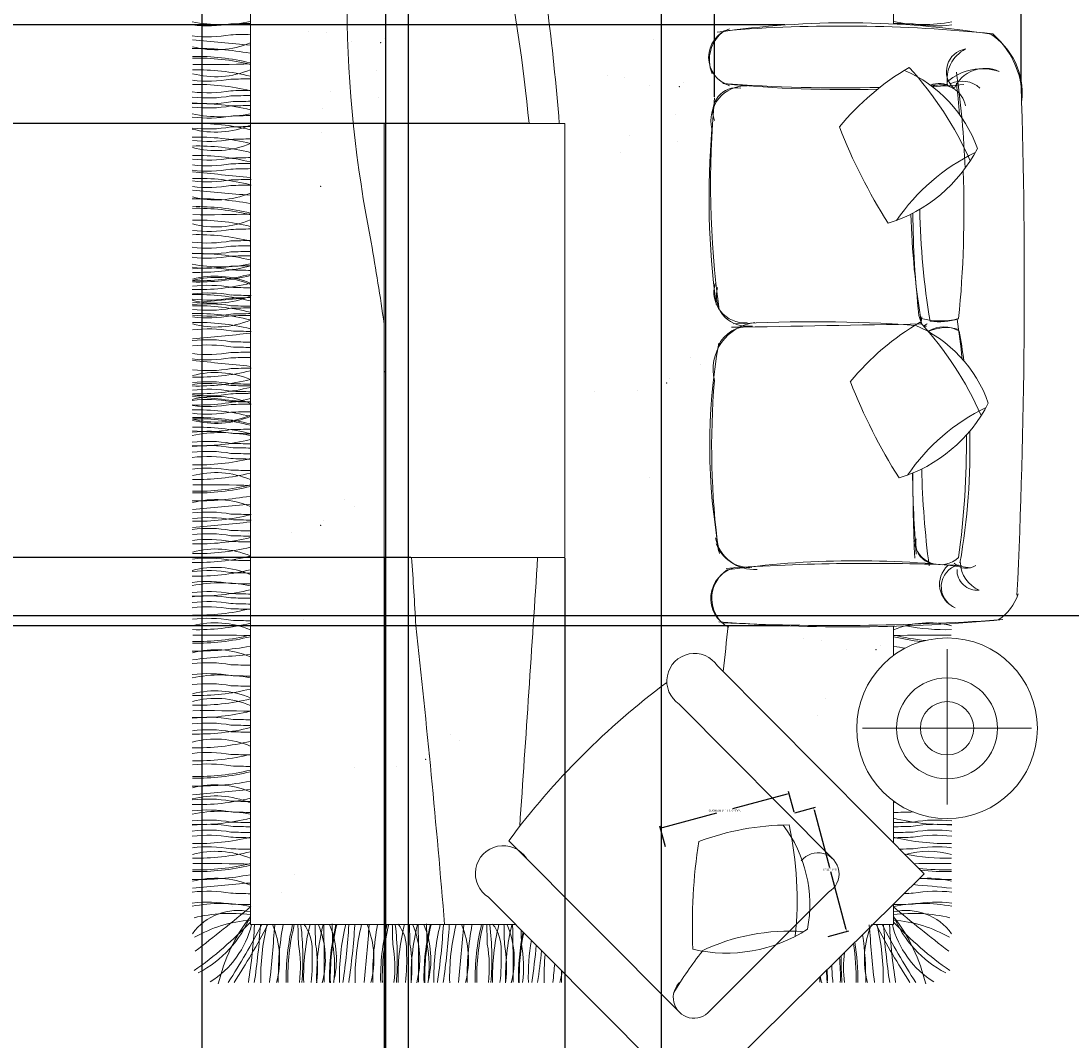
# Model space of a CAD drawing. Units: inches. Extents: x 503 to 1084, y -605 to 132.
# Tile 9 of 14: x 882 to 974, y -318 to -230. Entities that reach past the tile are written whole.
import ezdxf

# ---------------------------------------------------------------- set-up
doc = ezdxf.new("R2010")
doc.units = ezdxf.units.IN
doc.header["$MEASUREMENT"] = 0
doc.layers.add('A-ANNO-DIMS', color=7, linetype='Continuous', lineweight=18)
doc.layers.add('furniture', color=50, linetype='Continuous', lineweight=13, transparency=0.8)
doc.styles.get("Standard").update_dxf_attribs({"font": 'arial.ttf'})
doc.dimstyles.get("Standard").update_dxf_attribs({"dimtxt": 0.18, "dimasz": 0.18, "dimexe": 0.18, "dimexo": 0.0625, "dimgap": 0.09, "dimtad": 0, "dimtih": 1, "dimtoh": 1, "dimdec": 1, "dimzin": 0, "dimdsep": 46, "dimlunit": 4, "dimtxsty": 'Standard', "dimcen": 0.09, "dimadec": 0, "dimazin": 0, "dimtfac": 1, "dimtdec": 1, "dimtofl": 0, "dimtmove": 0, "dimatfit": 3, "dimfxl": 1, "dimtolj": 1, "dimtzin": 0, "dimarcsym": 0})

# ---------------------------------------------------------------- blocks, each defined once
blk = doc.blocks.new('CUSHION-SCATTER')
for centre, radius, start, end in [((-0.355, -5.979), 11.599, 64.45006, 111.76991), ((17.467, -0.489), 22.747, 165.30685, 185.5663), ((-5.995, -25.402), 30.717, 69.08153, 87.27682), ((-7.72, 0.481), 12.999, 332.0126, 17.9429), ((21.395, -1.669), 17.594, 160.90051, 190.65125), ((14.361, 41.881), 48.668, 246.33709, 257.41765)]:
    blk.add_arc(centre, radius, start, end)
blk = doc.blocks.new('*D30')
at = {"layer": 'A-ANNO-DIMS', "color": 0, "lineweight": -2, "transparency": 16777216}
for p, q in [((949.077, -296.859), (944.325, -298.132)), ((949.685, -298.435), (949.204, -296.639)), ((938.207, -299.772), (942.958, -298.499)), ((938.468, -301.441), (937.986, -299.645))]:
    blk.add_line(p, q, dxfattribs=at)
at = {"layer": 'A-ANNO-DIMS', "color": 0, "transparency": 16777216}
for points in [[(949.069, -296.83), (949.084, -296.888), (949.251, -296.813)], [(938.199, -299.743), (938.214, -299.801), (938.033, -299.818)]]:
    blk.add_solid(points, dxfattribs=at)
at = {"layer": 'Defpoints', "color": 0, "transparency": 16777216}
for p in [(949.251, -296.813), (949.701, -298.495), (938.484, -301.501)]:
    blk.add_point(p, dxfattribs=at)
at = {"layer": 'A-ANNO-DIMS', "color": 0, "transparency": 16777216, "insert": (943.642, -298.315), "char_height": 0.18, "attachment_point": 5}
blk.add_mtext('\\A1;CUSHION 0\'-11 1/2" TYP.', dxfattribs=at)
blk = doc.blocks.new('*D31')
at = {"layer": 'A-ANNO-DIMS', "color": 0, "lineweight": -2, "transparency": 16777216}
for p, q in [((949.762, -298.479), (951.558, -297.998)), ((951.431, -298.218), (952.78, -303.255)), ((954.227, -308.655), (952.878, -303.618)), ((952.651, -309.263), (954.448, -308.782))]:
    blk.add_line(p, q, dxfattribs=at)
at = {"layer": 'A-ANNO-DIMS', "color": 0, "transparency": 16777216}
for points in [[(951.46, -298.211), (951.402, -298.226), (951.384, -298.044)], [(954.256, -308.647), (954.198, -308.663), (954.274, -308.829)]]:
    blk.add_solid(points, dxfattribs=at)
at = {"layer": 'Defpoints', "color": 0, "transparency": 16777216}
for p in [(949.701, -298.495), (954.274, -308.829), (952.591, -309.279)]:
    blk.add_point(p, dxfattribs=at)
at = {"layer": 'A-ANNO-DIMS', "color": 0, "transparency": 16777216, "insert": (952.829, -303.437), "char_height": 0.18, "attachment_point": 5}
blk.add_mtext('\\A1;0\'-11" TYP.', dxfattribs=at)
blk = doc.blocks.new('*D45')
at = {"layer": 'A-ANNO-DIMS', "color": 0, "lineweight": -2, "transparency": 16777216}
for p, q in [((844.089, -354.753), (844.089, 43.514)), ((844.269, 43.334), (879.759, 43.334)), ((915.909, 43.334), (880.418, 43.334)), ((916.089, -354.753), (916.089, 43.514))]:
    blk.add_line(p, q, dxfattribs=at)
at = {"layer": 'A-ANNO-DIMS', "color": 0, "transparency": 16777216}
for points in [[(844.269, 43.364), (844.269, 43.304), (844.089, 43.334)], [(915.909, 43.364), (915.909, 43.304), (916.089, 43.334)]]:
    blk.add_solid(points, dxfattribs=at)
at = {"layer": 'Defpoints', "color": 0, "transparency": 16777216}
for p in [(916.089, 43.334), (844.089, -354.816), (916.089, -354.816)]:
    blk.add_point(p, dxfattribs=at)
at = {"layer": 'A-ANNO-DIMS', "color": 0, "transparency": 16777216, "insert": (880.089, 43.334), "char_height": 0.18, "attachment_point": 5}
blk.add_mtext('\\A1;6\'-0"', dxfattribs=at)
blk = doc.blocks.new('*D63')
at = {"layer": 'A-ANNO-DIMS', "color": 0, "lineweight": -2, "transparency": 16777216}
for p, q in [((783.151, -281.316), (1083.419, -281.316)), ((1083.239, -281.496), (1083.239, -317.883)), ((1083.239, -354.636), (1083.239, -318.249)), ((783.151, -354.816), (1083.419, -354.816))]:
    blk.add_line(p, q, dxfattribs=at)
at = {"layer": 'A-ANNO-DIMS', "color": 0, "transparency": 16777216}
for points in [[(1083.209, -281.496), (1083.269, -281.496), (1083.239, -281.316)], [(1083.209, -354.636), (1083.269, -354.636), (1083.239, -354.816)]]:
    blk.add_solid(points, dxfattribs=at)
at = {"layer": 'Defpoints', "color": 0, "transparency": 16777216}
for p in [(783.089, -281.316), (783.089, -354.816), (1083.239, -354.816)]:
    blk.add_point(p, dxfattribs=at)
at = {"layer": 'A-ANNO-DIMS', "color": 0, "transparency": 16777216, "insert": (1083.239, -318.066), "char_height": 0.18, "attachment_point": 5}
blk.add_mtext('\\A1;6\'-1 1/2"', dxfattribs=at)
blk = doc.blocks.new('*D64')
at = {"layer": 'A-ANNO-DIMS', "color": 0, "lineweight": -2, "transparency": 16777216}
for p, q in [((938.089, -162.878), (938.089, -583.146)), ((977.089, -162.878), (977.089, -583.146)), ((938.269, -582.966), (957.26, -582.966)), ((976.909, -582.966), (957.918, -582.966))]:
    blk.add_line(p, q, dxfattribs=at)
at = {"layer": 'A-ANNO-DIMS', "color": 0, "transparency": 16777216}
for points in [[(938.269, -582.936), (938.269, -582.996), (938.089, -582.966)], [(976.909, -582.936), (976.909, -582.996), (977.089, -582.966)]]:
    blk.add_solid(points, dxfattribs=at)
at = {"layer": 'Defpoints', "color": 0, "transparency": 16777216}
for p in [(938.089, -162.816), (977.089, -162.816), (977.089, -582.966)]:
    blk.add_point(p, dxfattribs=at)
at = {"layer": 'A-ANNO-DIMS', "color": 0, "transparency": 16777216, "insert": (957.589, -582.966), "char_height": 0.18, "attachment_point": 5}
blk.add_mtext('\\A1;3\'-3"', dxfattribs=at)
blk = doc.blocks.new('*D65')
at = {"layer": 'A-ANNO-DIMS', "color": 0, "lineweight": -2, "transparency": 16777216}
for p, q in [((898.089, -162.878), (898.089, -583.146)), ((914.089, -162.878), (914.089, -583.146)), ((898.269, -582.966), (905.768, -582.966)), ((913.909, -582.966), (906.409, -582.966))]:
    blk.add_line(p, q, dxfattribs=at)
at = {"layer": 'A-ANNO-DIMS', "color": 0, "transparency": 16777216}
for points in [[(898.269, -582.936), (898.269, -582.996), (898.089, -582.966)], [(913.909, -582.936), (913.909, -582.996), (914.089, -582.966)]]:
    blk.add_solid(points, dxfattribs=at)
at = {"layer": 'Defpoints', "color": 0, "transparency": 16777216}
for p in [(898.089, -162.816), (914.089, -162.816), (914.089, -582.966)]:
    blk.add_point(p, dxfattribs=at)
at = {"layer": 'A-ANNO-DIMS', "color": 0, "transparency": 16777216, "insert": (906.089, -582.966), "char_height": 0.18, "attachment_point": 5}
blk.add_mtext('\\A1;1\'-4"', dxfattribs=at)
blk = doc.blocks.new('*D71')
at = {"layer": 'A-ANNO-DIMS', "color": 0, "lineweight": -2, "transparency": 16777216}
for p, q in [((942.746, -236.149), (942.746, 43.514)), ((942.926, 43.334), (955.566, 43.334)), ((969.287, 43.334), (956.647, 43.334)), ((969.467, -235.109), (969.467, 43.514))]:
    blk.add_line(p, q, dxfattribs=at)
at = {"layer": 'A-ANNO-DIMS', "color": 0, "transparency": 16777216}
for points in [[(942.926, 43.364), (942.926, 43.304), (942.746, 43.334)], [(969.287, 43.364), (969.287, 43.304), (969.467, 43.334)]]:
    blk.add_solid(points, dxfattribs=at)
at = {"layer": 'Defpoints', "color": 0, "transparency": 16777216}
for p in [(969.467, 43.334), (969.467, -235.171), (942.746, -236.212)]:
    blk.add_point(p, dxfattribs=at)
at = {"layer": 'A-ANNO-DIMS', "color": 0, "transparency": 16777216, "insert": (956.106, 43.334), "char_height": 0.18, "attachment_point": 5}
blk.add_mtext('\\A1;2\'-2 1/2"', dxfattribs=at)
blk = doc.blocks.new('*D72')
at = {"layer": 'A-ANNO-DIMS', "color": 0, "lineweight": -2, "transparency": 16777216}
for p, q in [((948.886, -229.873), (552.759, -229.873)), ((552.939, -230.053), (552.939, -255.858)), ((552.939, -282.029), (552.939, -256.224)), ((949.25, -282.209), (552.759, -282.209))]:
    blk.add_line(p, q, dxfattribs=at)
at = {"layer": 'A-ANNO-DIMS', "color": 0, "transparency": 16777216}
for points in [[(552.909, -230.053), (552.969, -230.053), (552.939, -229.873)], [(552.909, -282.029), (552.969, -282.029), (552.939, -282.209)]]:
    blk.add_solid(points, dxfattribs=at)
at = {"layer": 'Defpoints', "color": 0, "transparency": 16777216}
for p in [(948.949, -229.873), (552.939, -282.209), (949.313, -282.209)]:
    blk.add_point(p, dxfattribs=at)
at = {"layer": 'A-ANNO-DIMS', "color": 0, "transparency": 16777216, "insert": (552.939, -256.041), "char_height": 0.18, "attachment_point": 5}
blk.add_mtext('\\A1;4\'-4 1/2"', dxfattribs=at)
blk = doc.blocks.new('*D77')
at = {"layer": 'A-ANNO-DIMS', "color": 0, "lineweight": -2, "transparency": 16777216}
for p, q in [((926.528, -238.468), (552.759, -238.468)), ((552.939, -238.648), (552.939, -257.175)), ((552.939, -276.066), (552.939, -257.539)), ((916.284, -276.246), (552.759, -276.246))]:
    blk.add_line(p, q, dxfattribs=at)
at = {"layer": 'A-ANNO-DIMS', "color": 0, "transparency": 16777216}
for points in [[(552.909, -238.648), (552.969, -238.648), (552.939, -238.468)], [(552.909, -276.066), (552.969, -276.066), (552.939, -276.246)]]:
    blk.add_solid(points, dxfattribs=at)
at = {"layer": 'Defpoints', "color": 0, "transparency": 16777216}
for p in [(926.59, -238.468), (552.939, -276.246), (916.347, -276.246)]:
    blk.add_point(p, dxfattribs=at)
at = {"layer": 'A-ANNO-DIMS', "color": 0, "transparency": 16777216, "insert": (552.939, -257.357), "char_height": 0.18, "attachment_point": 5}
blk.add_mtext('\\A1;3\'-2"', dxfattribs=at)
blk = doc.blocks.new('*D78')
at = {"layer": 'A-ANNO-DIMS', "color": 0, "lineweight": -2, "transparency": 16777216}
for p, q in [((913.968, -276.309), (913.968, -583.146)), ((929.709, -276.309), (929.709, -583.146)), ((914.148, -582.966), (921.308, -582.966)), ((929.529, -582.966), (922.369, -582.966))]:
    blk.add_line(p, q, dxfattribs=at)
at = {"layer": 'A-ANNO-DIMS', "color": 0, "transparency": 16777216}
for points in [[(914.148, -582.936), (914.148, -582.996), (913.968, -582.966)], [(929.529, -582.936), (929.529, -582.996), (929.709, -582.966)]]:
    blk.add_solid(points, dxfattribs=at)
at = {"layer": 'Defpoints', "color": 0, "transparency": 16777216}
for p in [(913.968, -276.246), (929.709, -276.246), (929.709, -582.966)]:
    blk.add_point(p, dxfattribs=at)
at = {"layer": 'A-ANNO-DIMS', "color": 0, "transparency": 16777216, "insert": (921.838, -582.966), "char_height": 0.18, "attachment_point": 5}
blk.add_mtext('\\A1;1\'-3 1/2"', dxfattribs=at)

msp = doc.modelspace()

# ---------------------------------------------------------------- linework, layer by layer
at = {"layer": 'furniture'}
for p, q in [((902.315, -308.222), (902.315, -208.108)), ((958.353, -211.41), (958.353, -229.789)), ((902.315, -223.932), (902.315, -308.222)), ((907.388, -230.457), (907.388, -230.457)), ((908.909, -230.574), (908.909, -230.574)), ((911.089, -231.349), (911.089, -231.349)), ((914.028, -231.06), (914.028, -231.06)), ((937.394, -231.145), (937.394, -231.145)), ((913.303, -233.845), (913.303, -233.845)), ((933.4, -234.298), (933.4, -234.298)), ((934.921, -234.415), (934.921, -234.415)), ((940.039, -234.901), (940.039, -234.901)), ((909.306, -235.668), (909.306, -235.668)), ((937.101, -235.19), (937.101, -235.19)), ((913.505, -236.221), (913.505, -236.221)), ((908.583, -237.163), (908.583, -237.163)), ((939.314, -237.685), (939.314, -237.685)), ((913.968, -238.468), (929.709, -238.468)), ((913.968, -276.246), (913.968, -238.468)), ((929.709, -238.468), (929.709, -276.246)), ((908.547, -239.233), (908.547, -239.233)), ((935.318, -239.509), (935.318, -239.509)), ((939.516, -240.062), (939.516, -240.062)), ((934.595, -241.003), (934.595, -241.003)), ((900.735, -251.062), (900.735, -251.062)), ((900.735, -251.173), (900.735, -251.173)), ((900.735, -254.588), (900.735, -254.588)), ((940.693, -258.862), (940.693, -258.862)), ((940.693, -258.862), (940.693, -258.862)), ((941.516, -259.407), (941.516, -259.407)), ((941.516, -259.407), (941.516, -259.407)), ((938.812, -260.625), (938.812, -260.625)), ((900.735, -261.742), (900.735, -261.742)), ((932.333, -261.767), (932.333, -261.767)), ((936.066, -261.711), (936.066, -261.711)), ((900.735, -265.157), (900.735, -265.157)), ((900.735, -265.268), (900.735, -265.268)), ((937.068, -269.297), (937.068, -269.297)), ((910.545, -271.248), (910.545, -271.248)), ((910.545, -271.248), (910.545, -271.248)), ((911.368, -271.793), (911.368, -271.793)), ((911.368, -271.793), (911.368, -271.793)), ((908.663, -273.011), (908.663, -273.011)), ((902.185, -274.153), (902.185, -274.153)), ((905.918, -274.097), (905.918, -274.097)), ((929.709, -276.246), (913.968, -276.246)), ((906.919, -281.683), (906.919, -281.683)), ((958.353, -282.247), (958.353, -284.782)), ((950.544, -283.34), (950.544, -283.34)), ((952.065, -283.458), (952.065, -283.458)), ((954.245, -284.232), (954.245, -284.232)), ((957.183, -283.943), (957.183, -283.943)), ((963.01, -291.127), (963.01, -284.237)), ((961.008, -303.791), (943.01, -285.687)), ((953.063, -302.511), (939.67, -289.026)), ((952.462, -288.552), (952.462, -288.552)), ((951.739, -290.046), (951.739, -290.046)), ((919.708, -291.633), (919.708, -291.633)), ((919.708, -291.633), (919.708, -291.633)), ((963.01, -291.127), (955.639, -291.127)), ((963.01, -291.127), (963.01, -297.761)), ((963.01, -291.127), (970.381, -291.127)), ((920.531, -292.178), (920.531, -292.178)), ((920.531, -292.178), (920.531, -292.178)), ((917.826, -293.396), (917.826, -293.396)), ((911.348, -294.538), (911.348, -294.538)), ((915.081, -294.482), (915.081, -294.482)), ((958.353, -297.472), (958.353, -301.12)), ((924.828, -300.918), (939.689, -315.851)), ((916.082, -302.069), (916.082, -302.069)), ((906.12, -303.883), (906.12, -303.883)), ((961.008, -303.791), (940.842, -323.704)), ((901.032, -305.419), (901.032, -305.419)), ((901.032, -305.419), (901.032, -305.419)), ((901.032, -305.419), (901.032, -305.419)), ((905.046, -305.391), (905.046, -305.391)), ((952.695, -305.393), (942.35, -315.738)), ((952.695, -305.393), (951.036, -307.051)), ((959.636, -305.419), (959.636, -305.419)), ((959.636, -305.419), (959.636, -305.419)), ((959.636, -305.419), (959.636, -305.419)), ((940.842, -323.704), (923.073, -305.836)), ((958.353, -306.412), (958.353, -308.222)), ((900.735, -306.63), (900.735, -306.63)), ((900.735, -306.63), (900.735, -306.63)), ((900.735, -306.63), (900.735, -306.63)), ((959.933, -306.63), (959.933, -306.63)), ((959.933, -306.63), (959.933, -306.63)), ((959.933, -306.63), (959.933, -306.63)), ((925.445, -308.222), (902.315, -308.222)), ((958.353, -308.222), (956.521, -308.222)), ((948.119, -309.968), (942.35, -315.738)), ((909.88, -310.915), (909.88, -310.915)), ((918.104, -310.915), (918.104, -310.915)), ((926.337, -310.915), (926.337, -310.915)), ((909.841, -311.391), (909.841, -311.391)), ((918.065, -311.391), (918.065, -311.391)), ((926.297, -311.391), (926.297, -311.391))]:
    msp.add_line(p, q, dxfattribs=at)
for radius in [7.871, 4.394, 2.321]:
    msp.add_circle((963.01, -291.127), radius, dxfattribs=at)
for centre, radius, start, end in [((1020.854, -227.369), 110.128, 169.92753, 191.22459), ((779.545, -252.476), 147.711, 5.44209, 17.47988), ((701.097, -256.901), 228.874, 4.61959, 9.75131), ((899.741, -217.088), 12.757, 258.75453, 281.58879), ((960.927, -217.088), 12.757, 258.41121, 281.24547), ((898.614, -218.573), 11.387, 263.11705, 280.06509), ((904.618, -356.744), 127.023, 91.02248, 91.81091), ((944.836, -232.692), 2.597, 107.71573, 252.84284), ((945.439, -232.917), 3.136, 126.0678, 202.6723), ((954.353, -307.898), 78.212, 80.80787, 98.3514), ((953.844, -357.089), 127.12, 84.0627, 94.62528), ((956.05, -356.744), 127.023, 88.18909, 88.97752), ((962.054, -218.573), 11.387, 259.93491, 276.88295), ((898.612, -219.524), 11.387, 263.11705, 280.06509), ((899.284, -224.175), 7.865, 255.13868, 292.69016), ((919.918, -8.385), 223.934, 264.19829, 265.48538), ((904.616, -357.695), 127.023, 91.02248, 91.81091), ((963.408, -235.789), 6.15, 353.87925, 57.10928), ((962.029, -236.303), 7.523, 8.65495, 48.71038), ((897.692, -257.399), 25.474, 79.59608, 90.98046), ((964.936, -233.922), 1.979, 99.29162, 227.62886), ((966.025, -234.636), 3.017, 117.84326, 189.86837), ((897.72, -251.804), 19.184, 76.14265, 91.36693), ((897.72, -251.947), 19.184, 76.14265, 91.36693), ((898.43, -69.087), 164.233, 269.60659, 271.37204), ((897.718, -252.972), 19.184, 76.14265, 91.36693), ((899.28, -226.519), 7.865, 255.13868, 292.69016), ((966.076, -238.311), 4.627, 71.24727, 131.13483), ((966.32, -236.582), 2.928, 64.87152, 156.7247), ((885.741, -245.387), 78.907, 2.2017, 8.30671), ((897.715, -254.241), 19.184, 76.14265, 91.36693), ((898.623, -223.392), 11.387, 263.11705, 280.06509), ((904.627, -361.563), 127.023, 91.02248, 91.81091), ((953.763, -94.836), 140.525, 265.80271, 271.38032), ((954.264, -119.888), 115.617, 264.74224, 271.33354), ((962.309, -236.968), 1.995, 57.73663, 112.23873), ((953.763, -94.836), 140.525, 273.19084, 273.78915), ((954.264, -119.888), 115.617, 273.71005, 275.06529), ((964.298, -237.104), 2.337, 47.72028, 114.44608), ((869.367, -246.113), 95.112, 5.08707, 6.74912), ((898.62, -224.398), 11.387, 263.11705, 280.06509), ((904.624, -362.57), 127.023, 91.02248, 91.81091), ((945.461, -238.198), 3.024, 87.65794, 194.09744), ((944.701, -237.434), 2.094, 80.26169, 201.01149), ((962.431, -237.331), 2.227, 10.62162, 109.19299), ((406.941, -252.727), 562.799, 357.2697, 1.7875), ((898.617, -225.352), 11.387, 263.11705, 280.06509), ((897.71, -255.891), 19.184, 76.14265, 91.36693), ((898.619, -224.849), 11.387, 263.11705, 280.06509), ((904.621, -363.892), 127.023, 91.02248, 91.81091), ((904.622, -363.523), 127.023, 91.02248, 91.81091), ((904.623, -363.02), 127.023, 91.02248, 91.81091), ((1024.621, -243.627), 82.21, 174.82447, 187.71479), ((898.614, -226.599), 11.387, 263.11705, 280.06509), ((898.616, -225.721), 11.387, 263.11705, 280.06509), ((899.741, -225.114), 12.757, 258.75453, 281.58879), ((904.618, -364.77), 127.023, 91.02248, 91.81091), ((897.706, -257.632), 19.184, 76.14265, 91.36693), ((899.267, -231.342), 7.865, 255.13868, 292.69016), ((904.616, -365.721), 127.023, 91.02248, 91.81091), ((898.612, -227.55), 11.387, 263.11705, 280.06509), ((897.708, -258.824), 19.184, 76.14265, 91.36693), ((1011.888, -244.908), 69.616, 175.07811, 187.69498), ((898.628, -228.63), 11.387, 263.11705, 280.06509), ((897.725, -259.599), 19.184, 76.14265, 91.36693), ((899.288, -232.95), 7.865, 255.13868, 292.69016), ((904.632, -366.802), 127.023, 91.02248, 91.81091), ((898.629, -230.259), 11.387, 263.11705, 280.06509), ((897.723, -260.437), 19.184, 76.14265, 91.36693), ((904.633, -368.431), 127.023, 91.02248, 91.81091), ((898.628, -230.762), 11.387, 263.11705, 280.06509), ((904.616, -369.393), 127.023, 91.02248, 91.81091), ((904.632, -368.933), 127.023, 91.02248, 91.81091), ((898.612, -231.222), 11.387, 263.11705, 280.06509), ((897.728, -262.419), 19.184, 76.14265, 91.36693), ((857.939, -666.7), 425.847, 84.01654, 84.69917), ((904.644, -370.33), 127.023, 91.02248, 91.81091), ((869.367, -246.113), 95.112, 354.36393, 2.12187), ((898.633, -232.648), 11.387, 263.11705, 280.06509), ((898.639, -232.158), 11.387, 263.11705, 280.06509), ((904.637, -370.82), 127.023, 91.02248, 91.81091), ((897.692, -270.48), 25.474, 79.59608, 90.98046), ((899.284, -237.257), 7.865, 255.13868, 292.69016), ((919.918, -21.467), 223.934, 264.19829, 265.48538), ((897.72, -264.885), 19.184, 76.14265, 91.36693), ((897.72, -265.028), 19.184, 76.14265, 91.36693), ((1025.867, -244.791), 65.245, 181.00607, 189.60009), ((897.718, -266.053), 19.184, 76.14265, 91.36693), ((899.28, -239.601), 7.865, 255.13868, 292.69016), ((898.43, -82.169), 164.233, 269.60659, 271.37204), ((1029.496, -244.355), 69.669, 181.64583, 189.52678), ((1047.624, -245.511), 87.597, 180.49489, 186.32914), ((898.623, -236.473), 11.387, 263.11705, 280.06509), ((904.627, -374.645), 127.023, 91.02248, 91.81091), ((898.62, -237.48), 11.387, 263.11705, 280.06509), ((897.715, -267.322), 19.184, 76.14265, 91.36693), ((904.624, -375.651), 127.023, 91.02248, 91.81091), ((702.149, -286.123), 213.963, 8.11901, 10.04424), ((898.617, -238.433), 11.387, 263.11705, 280.06509), ((898.619, -237.93), 11.387, 263.11705, 280.06509), ((904.622, -376.605), 127.023, 91.02248, 91.81091), ((904.623, -376.102), 127.023, 91.02248, 91.81091), ((898.616, -238.802), 11.387, 263.11705, 280.06509), ((897.71, -268.972), 19.184, 76.14265, 91.36693), ((904.621, -376.974), 127.023, 91.02248, 91.81091), ((898.614, -239.68), 11.387, 263.11705, 280.06509), ((899.741, -238.196), 12.757, 258.75453, 281.58879), ((898.629, -262.421), 11.387, 79.93491, 96.88295), ((897.723, -232.243), 19.184, 268.63307, 283.85735), ((904.618, -377.852), 127.023, 91.02248, 91.81091), ((904.633, -124.249), 127.023, 268.18909, 268.97752), ((897.708, -233.745), 19.184, 268.63307, 283.85735), ((897.725, -232.97), 19.184, 268.63307, 283.85735), ((897.725, -233.081), 19.184, 268.63307, 283.85735), ((899.288, -259.619), 7.865, 67.30984, 104.86132), ((899.288, -259.73), 7.865, 67.30984, 104.86132), ((945.347, -253.158), 2.651, 162.93165, 275.10915), ((897.706, -272.534), 19.184, 76.14265, 91.36693), ((898.628, -263.938), 11.387, 79.93491, 96.88295), ((898.639, -264.607), 11.387, 79.93491, 96.88295), ((904.632, -125.767), 127.023, 268.18909, 268.97752), ((904.644, -126.435), 127.023, 268.18909, 268.97752), ((945.537, -253.485), 2.627, 163.4437, 271.82282), ((898.612, -242.452), 11.387, 263.11705, 280.06509), ((898.612, -265.543), 11.387, 79.93491, 96.88295), ((899.267, -246.244), 7.865, 255.13868, 292.69016), ((857.939, 169.935), 425.847, 275.30083, 275.98346), ((904.616, -380.623), 127.023, 91.02248, 91.81091), ((897.708, -274.192), 19.184, 76.14265, 91.36693), ((898.628, -243.843), 11.387, 263.11705, 280.06509), ((898.628, -243.999), 11.387, 263.11705, 280.06509), ((898.629, -243.34), 11.387, 263.11705, 280.06509), ((897.723, -273.518), 19.184, 76.14265, 91.36693), ((904.616, -127.371), 127.023, 268.18909, 268.97752), ((904.632, -382.015), 127.023, 91.02248, 91.81091), ((904.632, -382.17), 127.023, 91.02248, 91.81091), ((904.633, -381.512), 127.023, 91.02248, 91.81091), ((933.975, -263.531), 27.871, 15.96247, 17.46375), ((897.725, -274.967), 19.184, 76.14265, 91.36693), ((899.288, -248.318), 7.865, 255.13868, 292.69016), ((946.732, -259.874), 4.101, 96.58671, 193.45107), ((945.783, -259.107), 2.995, 84.92344, 155.63742), ((-23769.776, 1386265.095), 1386741.544, 271.021158169, 271.0218453), ((951.391, -377.318), 121.599, 85.84252, 93.2873), ((962.425, -249.156), 6.497, 254.04794, 284.20605), ((1095.836, -269.752), 135.8, 173.88721, 174.12153), ((951.391, -377.318), 121.599, 85.36553, 85.4784), ((962.09, -257.334), 1.65, 119.13127, 132.01414), ((962.322, -250.391), 5.34, 261.53624, 288.34934), ((891.756, -266.303), 72.942, 5.77953, 8.52202), ((898.639, -267.737), 11.387, 79.93491, 96.88295), ((857.939, 166.805), 425.847, 275.30083, 275.98346), ((904.644, -129.565), 127.023, 268.18909, 268.97752), ((1040.559, -266.636), 79.781, 172.72451, 172.77255), ((962.91, -260.107), 3.873, 73.31083, 112.61636), ((962.717, -258.804), 2.632, 59.83188, 119.46797), ((908.309, -266.832), 56.697, 7.80299, 10.45572), ((898.612, -268.673), 11.387, 79.93491, 96.88295), ((898.628, -269.133), 11.387, 79.93491, 96.88295), ((904.616, -130.502), 127.023, 268.18909, 268.97752), ((904.632, -130.962), 127.023, 268.18909, 268.97752), ((994.188, -266.539), 51.852, 170.0543, 190.4167), ((898.612, -247.657), 11.387, 263.11705, 280.06509), ((898.628, -247.197), 11.387, 263.11705, 280.06509), ((904.616, -385.828), 127.023, 91.02248, 91.81091), ((904.632, -385.368), 127.023, 91.02248, 91.81091), ((857.939, -683.135), 425.847, 84.01654, 84.69917), ((904.644, -386.765), 127.023, 91.02248, 91.81091), ((897.725, -241.363), 19.184, 268.63307, 283.85735), ((899.288, -268.012), 7.865, 67.30984, 104.86132), ((898.639, -248.593), 11.387, 263.11705, 280.06509), ((897.708, -242.138), 19.184, 268.63307, 283.85735), ((898.628, -272.331), 11.387, 79.93491, 96.88295), ((898.628, -272.487), 11.387, 79.93491, 96.88295), ((898.629, -272.99), 11.387, 79.93491, 96.88295), ((897.723, -242.812), 19.184, 268.63307, 283.85735), ((904.632, -134.16), 127.023, 268.18909, 268.97752), ((904.632, -134.315), 127.023, 268.18909, 268.97752), ((1011.731, -266.613), 69.23, 175.20718, 187.55097), ((898.612, -250.787), 11.387, 263.11705, 280.06509), ((898.612, -273.878), 11.387, 79.93491, 96.88295), ((897.706, -243.796), 19.184, 268.63307, 283.85735), ((899.267, -270.086), 7.865, 67.30984, 104.86132), ((857.939, -686.265), 425.847, 84.01654, 84.69917), ((904.616, -388.959), 127.023, 91.02248, 91.81091), ((904.633, -134.818), 127.023, 268.18909, 268.97752), ((897.708, -282.585), 19.184, 76.14265, 91.36693), ((898.639, -251.724), 11.387, 263.11705, 280.06509), ((904.616, -135.707), 127.023, 268.18909, 268.97752), ((904.644, -389.895), 127.023, 91.02248, 91.81091), ((898.628, -252.392), 11.387, 263.11705, 280.06509), ((897.725, -283.249), 19.184, 76.14265, 91.36693), ((897.725, -283.36), 19.184, 76.14265, 91.36693), ((899.288, -256.6), 7.865, 255.13868, 292.69016), ((899.288, -256.711), 7.865, 255.13868, 292.69016), ((904.632, -390.563), 127.023, 91.02248, 91.81091), ((898.614, -276.65), 11.387, 79.93491, 96.88295), ((898.629, -253.909), 11.387, 263.11705, 280.06509), ((897.723, -284.087), 19.184, 76.14265, 91.36693), ((904.633, -392.081), 127.023, 91.02248, 91.81091), ((908.309, -266.832), 56.697, 349.94664, 1.59031), ((898.616, -277.528), 11.387, 79.93491, 96.88295), ((897.71, -247.358), 19.184, 268.63307, 283.85735), ((899.741, -278.134), 12.757, 78.41121, 101.24547), ((904.618, -138.478), 127.023, 268.18909, 268.97752), ((891.756, -266.303), 72.942, 352.15508, 0.55852), ((898.617, -277.897), 11.387, 79.93491, 96.88295), ((898.619, -278.4), 11.387, 79.93491, 96.88295), ((904.621, -139.356), 127.023, 268.18909, 268.97752), ((904.622, -139.725), 127.023, 268.18909, 268.97752), ((898.62, -278.85), 11.387, 79.93491, 96.88295), ((897.715, -249.008), 19.184, 268.63307, 283.85735), ((904.623, -140.228), 127.023, 268.18909, 268.97752), ((904.624, -140.679), 127.023, 268.18909, 268.97752), ((898.623, -279.857), 11.387, 79.93491, 96.88295), ((897.718, -250.277), 19.184, 268.63307, 283.85735), ((899.28, -276.729), 7.865, 67.30984, 104.86132), ((904.627, -141.685), 127.023, 268.18909, 268.97752), ((1069.195, -267.488), 109.199, 180.7456, 184.45597), ((1095.836, -269.752), 135.8, 179.63856, 182.76525), ((1040.559, -266.636), 79.781, 181.37312, 187.44721), ((897.72, -251.302), 19.184, 268.63307, 283.85735), ((897.72, -251.445), 19.184, 268.63307, 283.85735), ((898.43, -434.161), 164.233, 88.62796, 90.39341), ((897.692, -245.85), 25.474, 269.01954, 280.40392), ((899.284, -279.073), 7.865, 67.30984, 104.86132), ((919.918, -494.863), 223.934, 94.51462, 95.80171), ((898.633, -283.682), 11.387, 79.93491, 96.88295), ((897.728, -253.911), 19.184, 268.63307, 283.85735), ((904.637, -145.51), 127.023, 268.18909, 268.97752), ((898.639, -284.172), 11.387, 79.93491, 96.88295), ((857.939, 150.37), 425.847, 275.30083, 275.98346), ((904.644, -146), 127.023, 268.18909, 268.97752), ((898.612, -285.108), 11.387, 79.93491, 96.88295), ((898.628, -285.568), 11.387, 79.93491, 96.88295), ((904.616, -146.937), 127.023, 268.18909, 268.97752), ((904.632, -147.397), 127.023, 268.18909, 268.97752), ((898.629, -286.071), 11.387, 79.93491, 96.88295), ((897.723, -255.893), 19.184, 268.63307, 283.85735), ((904.633, -147.9), 127.023, 268.18909, 268.97752), ((946.184, -273.896), 3.406, 190.97559, 274.97468), ((945.867, -273.991), 3.153, 199.82281, 272.49854), ((962.432, -274.568), 2.317, 186.1174, 313.1189), ((962.112, -275.01), 1.835, 167.62255, 260.30943), ((897.708, -257.506), 19.184, 268.63307, 283.85735), ((897.725, -256.731), 19.184, 268.63307, 283.85735), ((899.288, -283.38), 7.865, 67.30984, 104.86132), ((715.469, -291.988), 201.494, 2.78771, 4.48071), ((-3564.101, 11.787), 4500.667, 356.03178, 356.330686), ((899.267, -284.988), 7.865, 67.30984, 104.86132), ((898.628, -287.7), 11.387, 79.93491, 96.88295), ((904.632, -149.528), 127.023, 268.18909, 268.97752), ((945.212, -279.819), 2.784, 104.63788, 244.30948), ((956.341, -458.74), 181.973, 87.50734, 93.9592), ((955.145, -357.728), 81.187, 82.98362, 97.98903), ((964.573, -278.588), 2.215, 132.31343, 247.61024), ((964.482, -278.81), 1.975, 104.78136, 247.59217), ((964.696, -275.707), 1.492, 224.39377, 303.58565), ((966.817, -276.647), 2.64, 181.18396, 247.82163), ((898.612, -288.78), 11.387, 79.93491, 96.88295), ((897.706, -258.698), 19.184, 268.63307, 283.85735), ((904.616, -150.609), 127.023, 268.18909, 268.97752), ((945.479, -279.815), 2.967, 123.04105, 226.06525), ((965.621, -277.36), 1.744, 178.0108, 276.55846), ((898.614, -289.731), 11.387, 79.93491, 96.88295), ((899.741, -291.216), 12.757, 78.41121, 101.24547), ((904.618, -151.56), 127.023, 268.18909, 268.97752), ((898.616, -290.609), 11.387, 79.93491, 96.88295), ((897.71, -260.439), 19.184, 268.63307, 283.85735), ((898.617, -290.978), 11.387, 79.93491, 96.88295), ((904.621, -152.438), 127.023, 268.18909, 268.97752), ((904.622, -152.807), 127.023, 268.18909, 268.97752), ((965.373, -278.315), 3.975, 301.88171, 343.96721), ((898.619, -291.481), 11.387, 79.93491, 96.88295), ((898.62, -291.932), 11.387, 79.93491, 96.88295), ((897.715, -262.089), 19.184, 268.63307, 283.85735), ((904.623, -153.31), 127.023, 268.18909, 268.97752), ((904.624, -153.76), 127.023, 268.18909, 268.97752), ((898.623, -292.938), 11.387, 79.93491, 96.88295), ((904.627, -154.767), 127.023, 268.18909, 268.97752), ((954.433, -140.354), 141.947, 265.43246, 275.43098), ((953.183, -73.845), 208.336, 267.31429, 273.93296), ((897.718, -263.358), 19.184, 268.63307, 283.85735), ((899.28, -289.811), 7.865, 67.30984, 104.86132), ((-7.273, -384.374), 929.631, 4.698728, 6.310761), ((1867.941, -384.374), 929.631, 173.689239, 173.937357), ((961.388, -289.811), 7.865, 75.13868, 112.69016), ((962.95, -263.358), 19.184, 259.37308, 271.36693), ((897.72, -264.383), 19.184, 268.63307, 283.85735), ((897.72, -264.526), 19.184, 268.63307, 283.85735), ((898.43, -447.243), 164.233, 88.62796, 90.39341), ((962.238, -447.243), 164.233, 89.60659, 91.37204), ((962.948, -264.526), 19.184, 256.14265, 263.44666), ((962.949, -264.383), 19.184, 256.14265, 264.58544), ((897.692, -258.931), 25.474, 269.01954, 280.40392), ((899.284, -292.155), 7.865, 67.30984, 104.86132), ((962.976, -258.931), 25.474, 259.59608, 261.86196), ((919.918, -507.945), 223.934, 94.51462, 95.80171), ((941.004, -287.021), 2.408, 33.6335, 236.3665), ((898.612, -296.806), 11.387, 79.93491, 96.88295), ((904.616, -158.635), 127.023, 268.18909, 268.97752), ((898.614, -297.758), 11.387, 79.93491, 96.88295), ((899.741, -299.242), 12.757, 78.41121, 101.24547), ((904.618, -159.586), 127.023, 268.18909, 268.97752), ((978.573, -340.839), 66.949, 126.66127, 143.39506), ((898.616, -298.635), 11.387, 79.93491, 96.88295), ((897.725, -269.085), 19.184, 268.63307, 283.85735), ((899.288, -295.734), 7.865, 67.30984, 104.86132), ((904.621, -160.464), 127.023, 268.18909, 268.97752), ((897.718, -269.942), 19.184, 268.63307, 283.85735), ((899.28, -296.395), 7.865, 67.30984, 104.86132), ((897.71, -271.018), 19.184, 268.63307, 283.85735), ((898.43, -453.826), 164.233, 88.62796, 90.39341), ((898.617, -301.557), 11.387, 79.93491, 96.88295), ((898.619, -302.06), 11.387, 79.93491, 96.88295), ((904.622, -163.385), 127.023, 268.18909, 268.97752), ((904.623, -163.888), 127.023, 268.18909, 268.97752), ((897.708, -272.449), 19.184, 268.63307, 283.85735), ((898.628, -302.642), 11.387, 79.93491, 96.88295), ((904.632, -164.471), 127.023, 268.18909, 268.97752), ((897.706, -273.641), 19.184, 268.63307, 283.85735), ((899.267, -299.931), 7.865, 67.30984, 104.86132), ((898.62, -304.618), 11.387, 79.93491, 96.88295), ((897.715, -274.776), 19.184, 268.63307, 283.85735), ((904.624, -166.447), 127.023, 268.18909, 268.97752), ((898.623, -305.625), 11.387, 79.93491, 96.88295), ((904.627, -167.453), 127.023, 268.18909, 268.97752), ((897.72, -276.145), 19.184, 268.63307, 283.85735), ((897.72, -276.288), 19.184, 268.63307, 283.85735), ((897.692, -270.693), 25.474, 269.01954, 280.40392), ((899.284, -303.917), 7.865, 67.30984, 104.86132), ((898.612, -308.679), 11.387, 79.93491, 96.88295), ((897.706, -278.597), 19.184, 268.63307, 283.85735), ((899.267, -304.887), 7.865, 67.30984, 104.86132), ((919.918, -519.707), 223.934, 94.51462, 95.80171), ((904.616, -170.508), 127.023, 268.18909, 268.97752), ((956.052, -170.508), 127.023, 271.02248, 271.06056), ((961.401, -304.887), 7.865, 111.65199, 112.69016), ((898.614, -309.63), 11.387, 79.93491, 96.88295), ((898.616, -310.508), 11.387, 79.93491, 96.88295), ((897.71, -280.338), 19.184, 268.63307, 283.85735), ((899.741, -311.115), 12.757, 78.41121, 101.24547), ((904.618, -171.459), 127.023, 268.18909, 268.97752), ((956.05, -171.459), 127.023, 271.02248, 271.81091), ((962.958, -280.338), 19.184, 256.14265, 271.36693), ((962.052, -310.508), 11.387, 83.11705, 100.06509), ((898.617, -310.877), 11.387, 79.93491, 96.88295), ((898.619, -311.38), 11.387, 79.93491, 96.88295), ((904.621, -172.337), 127.023, 268.18909, 268.97752), ((904.622, -172.706), 127.023, 268.18909, 268.97752), ((956.047, -172.706), 127.023, 271.02248, 271.81091), ((956.048, -172.337), 127.023, 271.02248, 271.81091), ((962.049, -311.38), 11.387, 83.11705, 100.06509), ((962.051, -310.877), 11.387, 83.11705, 100.06509), ((898.62, -311.831), 11.387, 79.93491, 96.88295), ((897.715, -281.988), 19.184, 268.63307, 283.85735), ((904.623, -173.209), 127.023, 268.18909, 268.97752), ((904.624, -173.659), 127.023, 268.18909, 268.97752), ((956.044, -173.659), 127.023, 271.02248, 271.81091), ((956.045, -173.209), 127.023, 271.02248, 271.81091), ((962.953, -281.988), 19.184, 256.14265, 271.36693), ((962.048, -311.831), 11.387, 83.11705, 100.06509), ((898.623, -312.837), 11.387, 79.93491, 96.88295), ((899.28, -309.71), 7.865, 67.30984, 104.86132), ((904.627, -174.666), 127.023, 268.18909, 268.97752), ((924.337, -303.771), 2.421, 33.09238, 238.53066), ((956.041, -174.666), 127.023, 271.2964, 271.81091), ((961.388, -309.71), 7.865, 75.13868, 104.83406), ((962.045, -312.837), 11.387, 83.11705, 100.06509), ((897.718, -283.257), 19.184, 268.63307, 283.85735), ((951.762, -303.809), 1.838, 300.48188, 142.32523), ((962.95, -283.257), 19.184, 259.25336, 271.36693), ((897.72, -284.282), 19.184, 268.63307, 283.85735), ((897.72, -284.425), 19.184, 268.63307, 283.85735), ((898.43, -467.142), 164.233, 88.62796, 90.39341), ((962.238, -467.142), 164.233, 89.60659, 90.73035), ((962.949, -284.282), 19.184, 262.7707, 271.36693), ((962.948, -284.425), 19.184, 263.2584, 271.36693), ((897.692, -278.83), 25.474, 269.01954, 280.40392), ((899.284, -312.054), 7.865, 67.30984, 104.86132), ((919.918, -527.844), 223.934, 94.51462, 95.80171), ((961.384, -312.054), 7.865, 75.13868, 96.00411), ((962.976, -278.83), 25.474, 264.64881, 270.98046), ((898.612, -316.705), 11.387, 79.93491, 96.88295), ((904.616, -178.534), 127.023, 268.18909, 268.97752), ((956.052, -178.534), 127.023, 271.46162, 271.81091), ((940.751, -527.844), 223.934, 84.19829, 85.05746), ((962.057, -316.705), 11.387, 83.11705, 100.06509), ((898.614, -317.657), 11.387, 79.93491, 96.88295), ((899.741, -319.141), 12.757, 78.41121, 101.24547), ((904.618, -179.485), 127.023, 268.18909, 268.97752), ((956.05, -179.485), 127.023, 271.02248, 271.81091), ((960.927, -319.141), 12.757, 78.75453, 101.58879), ((962.054, -317.657), 11.387, 83.11705, 100.06509), ((901.229, -311.893), 4.899, 77.19461, 144.09429), ((900.593, -321.089), 13.836, 82.85092, 103.27854), ((802.813, -187.345), 155.386, 307.54408, 309.84318), ((1057.855, -187.345), 155.386, 230.15682, 232.45592), ((959.439, -311.893), 4.899, 35.90571, 102.80539), ((960.075, -321.089), 13.836, 76.72146, 97.14908), ((877.858, -284.624), 33.837, 305.31527, 316.284), ((903.172, -319.304), 11.499, 94.27565, 119.86497), ((893.328, -303.809), 9.701, 297.30329, 337.88189), ((894.389, -306.225), 8.279, 302.27123, 346.00651), ((914.057, -316.74), 14.916, 141.9231, 167.04771), ((853.121, -282.36), 56.461, 326.82194, 332.73315), ((853.631, -282.373), 56.461, 326.82194, 332.73315), ((847.93, -305.036), 54.836, 351.37714, 356.63558), ((848.44, -305.049), 54.836, 351.37714, 356.63558), ((922.401, -312.826), 19.184, 166.14265, 181.36693), ((681.204, -290.619), 223.934, 354.19829, 355.48538), ((896.994, -311.253), 7.865, 345.13868, 22.69016), ((930.218, -312.845), 25.474, 169.59608, 180.98046), ((924.623, -312.817), 19.184, 166.14265, 181.36693), ((924.766, -312.817), 19.184, 166.14265, 181.36693), ((1033.458, -305.91), 127.023, 181.02248, 181.81091), ((880.977, -311.246), 25.914, 355.49364, 6.62982), ((926.135, -312.822), 19.184, 166.14265, 181.36693), ((904.267, -310.308), 3.43, 356.82563, 38.34356), ((1034.954, -305.915), 127.023, 181.02248, 181.81091), ((927.27, -312.831), 19.184, 166.14265, 181.36693), ((900.98, -311.269), 7.865, 345.13868, 22.69016), ((744.513, -312.107), 164.233, 359.60659, 1.37204), ((901.945, -311.256), 7.865, 345.13868, 22.69016), ((928.398, -312.819), 19.184, 166.14265, 181.36693), ((928.462, -312.829), 19.184, 166.14265, 181.36693), ((1036.44, -305.905), 127.023, 181.02248, 181.81091), ((929.255, -312.812), 19.184, 166.14265, 181.36693), ((856.154, -305.036), 54.836, 351.37714, 356.63558), ((856.664, -305.049), 54.836, 351.37714, 356.63558), ((930.624, -312.826), 19.184, 166.14265, 181.36693), ((689.428, -290.619), 223.934, 354.19829, 355.48538), ((905.218, -311.253), 7.865, 345.13868, 22.69016), ((938.442, -312.845), 25.474, 169.59608, 180.98046), ((932.847, -312.817), 19.184, 166.14265, 181.36693), ((932.99, -312.817), 19.184, 166.14265, 181.36693), ((1041.682, -305.91), 127.023, 181.02248, 181.81091), ((889.201, -311.246), 25.914, 355.49364, 6.62982), ((934.359, -312.822), 19.184, 166.14265, 181.36693), ((912.491, -310.308), 3.43, 356.82563, 38.34356), ((1043.178, -305.915), 127.023, 181.02248, 181.81091), ((935.494, -312.831), 19.184, 166.14265, 181.36693), ((909.204, -311.269), 7.865, 345.13868, 22.69016), ((752.737, -312.107), 164.233, 359.60659, 1.37204), ((910.169, -311.256), 7.865, 345.13868, 22.69016), ((936.622, -312.819), 19.184, 166.14265, 181.36693), ((936.686, -312.829), 19.184, 166.14265, 181.36693), ((1044.664, -305.905), 127.023, 181.02248, 181.81091), ((937.479, -312.812), 19.184, 166.14265, 181.36693), ((864.387, -305.036), 54.836, 351.37714, 356.63558), ((864.897, -305.049), 54.836, 351.37714, 356.63558), ((938.857, -312.826), 19.184, 166.14265, 181.36693), ((697.661, -290.619), 223.934, 354.19829, 355.48538), ((913.451, -311.253), 7.865, 345.13868, 22.69016), ((946.675, -312.845), 25.474, 169.59608, 180.98046), ((941.08, -312.817), 19.184, 166.14265, 181.36693), ((941.223, -312.817), 19.184, 166.14265, 181.36693), ((1049.914, -305.91), 127.023, 181.02248, 181.81091), ((897.434, -311.246), 25.914, 355.49364, 6.62982), ((942.592, -312.822), 19.184, 166.14265, 181.36693), ((920.724, -310.308), 3.43, 356.82563, 38.34356), ((1051.411, -305.915), 127.023, 181.02248, 181.81091), ((943.727, -312.831), 19.184, 166.14265, 181.36693), ((917.437, -311.269), 7.865, 345.13868, 22.69016), ((760.97, -312.107), 164.233, 359.60659, 1.37204), ((963.674, -311.253), 7.865, 157.30984, 194.86132), ((1179.464, -290.619), 223.934, 184.51462, 185.80171), ((1007.037, -282.373), 56.461, 207.26685, 213.17806), ((938.268, -312.826), 19.184, 358.63307, 13.85735), ((1007.547, -282.36), 56.461, 207.26685, 213.17806), ((1012.228, -305.049), 54.836, 183.36442, 188.62286), ((1012.738, -305.036), 54.836, 183.36442, 188.62286), ((966.279, -306.225), 8.279, 193.99349, 237.72877), ((967.34, -303.809), 9.701, 202.11811, 242.69671), ((946.611, -316.74), 14.916, 12.95229, 38.0769), ((957.496, -319.304), 11.499, 60.13503, 85.72435), ((982.81, -284.624), 33.837, 223.716, 234.68473), ((944.854, -312.819), 19.184, 168.09925, 181.36693), ((944.919, -312.829), 19.184, 168.23618, 181.36693), ((1052.897, -305.905), 127.023, 181.25348, 181.81091), ((930.45, -312.845), 25.474, 359.01954, 8.48469), ((895.286, -311.914), 11.387, 353.11705, 10.06509), ((896.783, -311.919), 11.387, 353.11705, 10.06509), ((898.269, -311.909), 11.387, 353.11705, 10.06509), ((903.51, -311.914), 11.387, 353.11705, 10.06509), ((905.007, -311.919), 11.387, 353.11705, 10.06509), ((906.493, -311.909), 11.387, 353.11705, 10.06509), ((911.743, -311.914), 11.387, 353.11705, 10.06509), ((913.24, -311.919), 11.387, 353.11705, 10.06509), ((914.725, -311.909), 11.387, 353.11705, 10.06509), ((945.711, -312.812), 19.184, 170.31586, 181.36693), ((872.611, -305.036), 54.836, 351.37714, 354.79861), ((935.902, -312.817), 19.184, 358.63307, 8.85609), ((936.045, -312.817), 19.184, 358.63307, 9.2236), ((889.96, -311.29), 17.75, 353.55867, 2.55652), ((898.184, -311.29), 17.75, 353.55867, 2.55652), ((906.417, -311.29), 17.75, 353.55867, 2.55652), ((873.121, -305.049), 54.836, 351.37714, 354.31935), ((947.081, -312.826), 19.184, 173.92295, 181.36693), ((969.526, -332.409), 35.395, 141.84571, 148.91333), ((979.691, -311.246), 25.914, 179.29867, 184.50636), ((965.382, -311.914), 11.387, 173.60686, 186.88295), ((705.885, -290.619), 223.934, 354.19829, 354.6171), ((970.708, -311.29), 17.75, 181.43318, 186.44133), ((934.533, -312.822), 19.184, 358.63307, 5.24223), ((921.675, -311.253), 7.865, 345.13868, 352.54782), ((954.898, -312.845), 25.474, 178.61905, 180.98046), ((1116.155, -312.107), 164.233, 180.22836, 180.39341), ((959.688, -311.269), 7.865, 190.67922, 194.86132), ((963.885, -311.919), 11.387, 181.36657, 186.88295), ((933.398, -312.831), 19.184, 358.63307, 2.11353), ((940.967, -314.574), 1.807, 130.10925, 319.89075)]:
    msp.add_arc(centre, radius, start, end, dxfattribs=at)
for p in [(913.678, -231.409), (939.69, -235.249), (908.445, -243.937), (914.024, -260.07), (938.572, -261.056), (908.423, -273.442), (956.834, -284.292), (917.586, -293.828)]:
    msp.add_point(p, dxfattribs=at)

# ---------------------------------------------------------------- block references
for p, rotation in [((959.193, -240.512), 314.9999999839699), ((960.147, -262.699), 314.9999999843537), ((945.317, -305.294), 284.9999999875181)]:
    msp.add_blockref('CUSHION-SCATTER', p, dxfattribs=dict(at, rotation=rotation))

# ---------------------------------------------------------------- dimensions: what is measured, and where the dimension line sits
at = {"layer": 'A-ANNO-DIMS'}
for base, p1, p2, picture, middle in [((916.089, 43.334), (844.089, -354.816), (916.089, -354.816), '*D45', (880.089, 43.334)), ((969.467, 43.334), (942.746, -236.212), (969.467, -235.171), '*D71', (956.106, 43.334)), ((914.089, -582.966), (898.089, -162.816), (914.089, -162.816), '*D65', (906.089, -582.966)), ((977.089, -582.966), (938.089, -162.816), (977.089, -162.816), '*D64', (957.589, -582.966)), ((929.709, -582.966), (913.968, -276.246), (929.709, -276.246), '*D78', (921.838, -582.966))]:
    dim = msp.add_linear_dim(base=base, p1=p1, p2=p2, dimstyle='Standard', override={"dimdec": 1, "dimlfac": 1, "dimrnd": 0, "dimzin": 1, "dimdsep": 46, "dimlunit": 4, "dimfrac": 2}, dxfattribs=at)
    dim.commit()
    dim.dimension.update_dxf_attribs({"geometry": picture, "text_midpoint": middle})
for base, p1, p2, picture, middle in [((552.939, -282.209), (948.949, -229.873), (949.313, -282.209), '*D72', (552.939, -256.041)), ((552.939, -276.246), (926.59, -238.468), (916.347, -276.246), '*D77', (552.939, -257.357)), ((1083.239, -354.816), (783.089, -281.316), (783.089, -354.816), '*D63', (1083.239, -318.066))]:
    dim = msp.add_linear_dim(base=base, p1=p1, p2=p2, angle=90, dimstyle='Standard', override={"dimdec": 1, "dimlfac": 1, "dimrnd": 0, "dimzin": 1, "dimdsep": 46, "dimlunit": 4, "dimfrac": 2}, dxfattribs=at)
    dim.commit()
    dim.dimension.update_dxf_attribs({"geometry": picture, "text_midpoint": middle})
for base, p1, p2, angle, text, picture, middle in [((949.251, -296.813), (938.484, -301.501), (949.701, -298.495), 15, 'CUSHION <> TYP.', '*D30', (943.642, -298.315)), ((954.274, -308.829), (949.701, -298.495), (952.591, -309.279), 285, '<> TYP.', '*D31', (952.829, -303.437))]:
    dim = msp.add_linear_dim(base=base, p1=p1, p2=p2, angle=angle, text=text, dimstyle='Standard', override={"dimdec": 1, "dimlfac": 1, "dimrnd": 0, "dimzin": 1, "dimdsep": 46, "dimlunit": 4, "dimfrac": 2}, dxfattribs=at)
    dim.commit()
    dim.dimension.update_dxf_attribs({"geometry": picture, "text_midpoint": middle})

doc.saveas('drawing.dxf')
